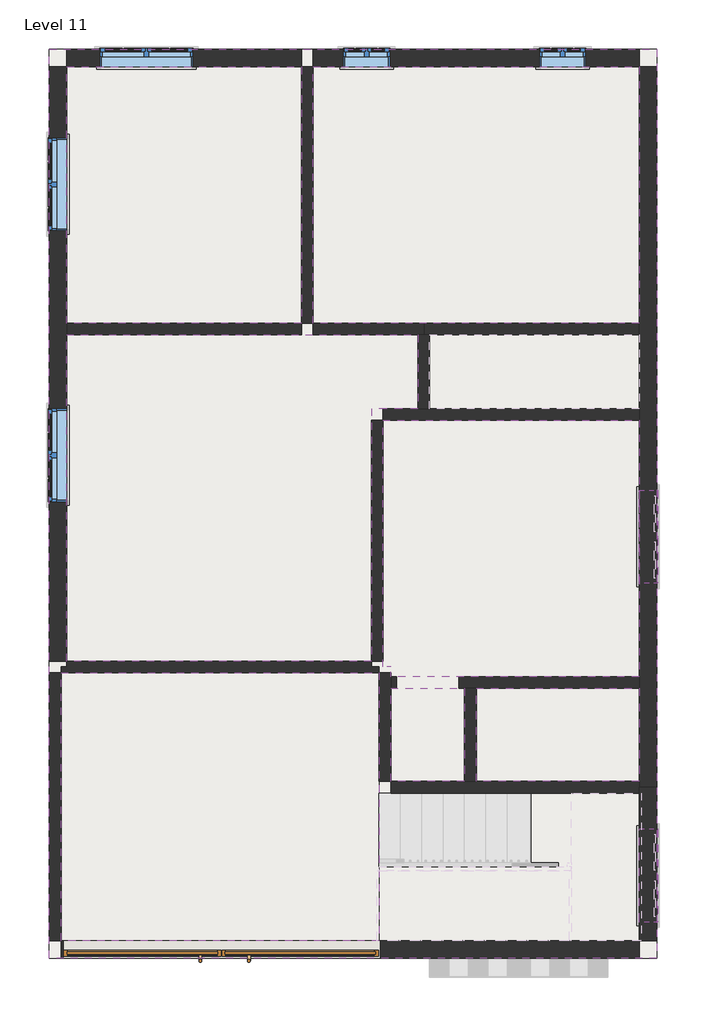
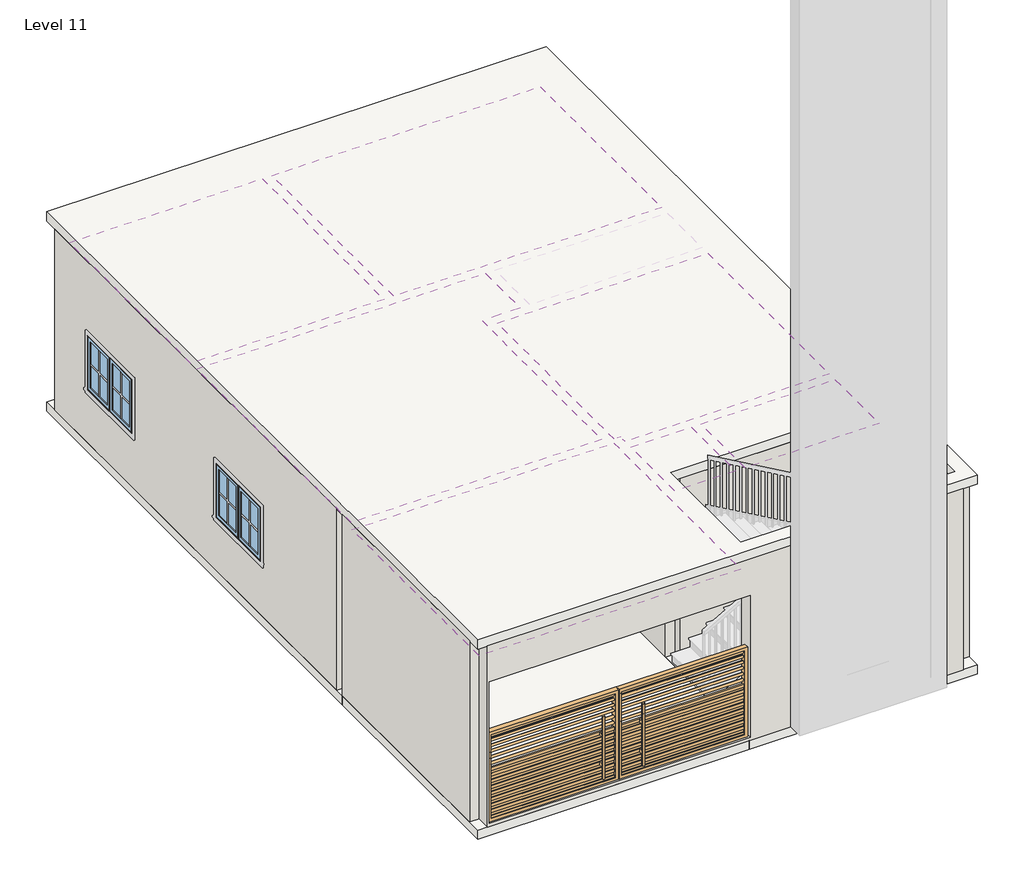
# One storey, part 1 of 3: 28 walls, 11 windows, 7 coverings, 3 slabs, 1 door.
"""IFC4 building model written with IfcOpenShell, lengths in millimetres."""

from ifc_helpers import new_model, si_unit, frame, origin, origin_with_axes, place, context, project, spatial, polyline, outline, extrude, faceted_brep, transform, mapped, element, save
from components import gate_gate_6d9155c2, window_casement_double_3_c417fced, window_casement_double_4_c19c33cb

model = new_model("IFC4")

# Units and contexts
model_context = context("Model", 3, world=origin())
ifc_project = project(units=[si_unit("LENGTHUNIT", "METRE", prefix="MILLI")], contexts=[model_context])

# Site, building, storey
site = spatial("IfcSite", under=ifc_project)
building = spatial("IfcBuilding", under=site)
storey = spatial("IfcBuildingStorey", under=building, Name="Level 11", Elevation=0.0)

# Coverings
placement = place(None, origin())
element("IfcCovering", 1, ObjectType="2' x 4' ACT System", at=placement, inside=storey, context=model_context, shape_type="SweptSolid", body=[
    extrude(outline(polyline([(-5680.5154463, 2323.8455275), (-5680.5154463, 5678.2330275), (-2607.1154463, 5678.2330275), (-2607.1154463, 2323.8455275), (-5680.5154463, 2323.8455275)])), frame((0.0, 0.0, 2743.2), z_axis=(0.0, 0.0, 1.0), x_axis=(1.0, 0.0, 0.0)), (0.0, 0.0, 1.0), 57.15),
])
element("IfcCovering", 2, ObjectType="2' x 4' ACT System", at=placement, inside=storey, context=model_context, shape_type="SweptSolid", body=[
    extrude(outline(polyline([(-2454.7154463, 2323.8455275), (-2454.7154463, 5678.2330275), (1812.4845537, 5678.2330275), (1812.4845537, 2323.8455275), (-2454.7154463, 2323.8455275)])), frame((0.0, 0.0, 2743.2), z_axis=(0.0, 0.0, 1.0), x_axis=(1.0, 0.0, 0.0)), (0.0, 0.0, 1.0), 57.15),
])
element("IfcCovering", 3, ObjectType="2' x 4' ACT System", at=placement, inside=storey, context=model_context, shape_type="SweptSolid", body=[
    extrude(outline(polyline([(-5680.5154463, -2095.7544725), (-5680.5154463, 2171.4455275), (-1083.1154463, 2171.4455275), (-1083.1154463, 1206.2455275), (-1692.7154463, 1206.2455275), (-1692.7154463, -2095.7544725), (-5680.5154463, -2095.7544725)])), frame((0.0, 0.0, 2743.2), z_axis=(0.0, 0.0, 1.0), x_axis=(1.0, 0.0, 0.0)), (0.0, 0.0, 1.0), 57.15),
])
element("IfcCovering", 4, ObjectType="2' x 4' ACT System", at=placement, inside=storey, context=model_context, shape_type="SweptSolid", body=[
    extrude(outline(polyline([(1812.4845537, 1053.8455275), (1812.4845537, -2298.9544725), (-1438.7154463, -2298.9544725), (-1438.7154463, -2171.9544725), (-1540.3154463, -2171.9544725), (-1540.3154463, 1053.8455275), (1812.4845537, 1053.8455275)])), frame((0.0, 0.0, 2743.2), z_axis=(0.0, 0.0, 1.0), x_axis=(1.0, 0.0, 0.0)), (0.0, 0.0, 1.0), 57.15),
])
element("IfcCovering", 5, ObjectType="2' x 4' ACT System", at=placement, inside=storey, context=model_context, shape_type="SweptSolid", body=[
    extrude(outline(polyline([(1812.4845537, -2451.3544725), (1812.4845537, -3670.5544725), (-321.1154463, -3670.5544725), (-321.1154463, -2451.3544725), (1812.4845537, -2451.3544725)])), frame((0.0, 0.0, 2743.2), z_axis=(0.0, 0.0, 1.0), x_axis=(1.0, 0.0, 0.0)), (0.0, 0.0, 1.0), 57.15),
])
element("IfcCovering", 6, ObjectType="2' x 4' ACT System", at=placement, inside=storey, context=model_context, shape_type="SweptSolid", body=[
    extrude(outline(polyline([(-473.5154463, -2451.3544725), (-473.5154463, -3670.5544725), (-1438.7154463, -3670.5544725), (-1438.7154463, -2451.3544725), (-473.5154463, -2451.3544725)])), frame((0.0, 0.0, 2743.2), z_axis=(0.0, 0.0, 1.0), x_axis=(1.0, 0.0, 0.0)), (0.0, 0.0, 1.0), 57.15),
])
element("IfcCovering", 7, ObjectType="2' x 4' ACT System", at=placement, inside=storey, context=model_context, shape_type="SweptSolid", body=[
    extrude(outline(polyline([(-1591.1154463, -2248.1544725), (-1591.1154463, -5753.3544725), (-5756.7154463, -5753.3544725), (-5756.7154463, -2248.1544725), (-1591.1154463, -2248.1544725)])), frame((0.0, 0.0, 2743.2), z_axis=(0.0, 0.0, 1.0), x_axis=(1.0, 0.0, 0.0)), (0.0, 0.0, 1.0), 57.15),
])

# Door
gate_gate_shape = gate_gate_6d9155c2(model_context)
element("IfcDoor", 8, ObjectType="GATE : GATE", at=placement, inside=storey, context=model_context, shape_type="MappedRepresentation", body=[
    mapped(gate_gate_shape, transform((0.0, 0.0, 0.0), x_axis=(1.0, 0.0, 0.0), y_axis=(0.0, 1.0, 0.0), z_axis=(0.0, 0.0, 1.0))),
])

# Slabs
element("IfcSlab", 9, ObjectType="Generic - 6\"", at=placement, inside=storey, context=model_context, shape_type="SweptSolid", body=[
    extrude(outline(polyline([(-5909.1154463, -2248.1544725), (-5909.1154463, 5906.8330275), (2041.0845537, 5906.8330275), (2041.0845537, -5981.9544725), (-1591.1154463, -5981.9544725), (-1591.1154463, -2248.1544725), (-5756.7154463, -2248.1544725), (-5909.1154463, -2248.1544725)])), frame((0.0, 0.0, -152.4), z_axis=(0.0, 0.0, 1.0), x_axis=(1.0, 0.0, 0.0)), (0.0, 0.0, 1.0), 152.4),
])
element("IfcSlab", 10, ObjectType="Generic - 6\"", at=placement, inside=storey, context=model_context, shape_type="SweptSolid", body=[
    extrude(outline(polyline([(-1591.1154463, -2248.1544725), (-1591.1154463, -5981.9544725), (-5909.1154463, -5981.9544725), (-5909.1154463, -2248.1544725), (-1591.1154463, -2248.1544725)])), frame((0.0, 0.0, -152.4), z_axis=(0.0, 0.0, 1.0), x_axis=(1.0, 0.0, 0.0)), (0.0, 0.0, 1.0), 152.4),
])
element("IfcSlab", 11, ObjectType="Generic - 6\"", at=placement, inside=storey, context=model_context, shape_type="SweptSolid", body=[
    extrude(outline(polyline([(2041.0845537, 5906.8330275), (2041.0845537, -5981.9544725), (-5909.1154463, -5981.9544725), (-5909.1154463, 5906.8330275), (2041.0845537, 5906.8330275)]), holes=[polyline([(1812.4845537, -3822.9544725), (-1591.1154463, -3822.9544725), (-1591.1154463, -5753.3544725), (1812.4845537, -5753.3544725), (1812.4845537, -3822.9544725)])]), frame((0.0, 0.0, 3048.0), z_axis=(0.0, 0.0, 1.0), x_axis=(1.0, 0.0, 0.0)), (0.0, 0.0, 1.0), 152.4),
])

# Walls
element("IfcWall", 12, ObjectType="Generic - 6\"", at=placement, inside=storey, context=model_context, shape_type="SweptSolid", body=[
    extrude(outline(polyline([(-5909.1154463, -5753.3544725), (-5909.1154463, -2248.1544725), (-5756.7154463, -2248.1544725), (-5756.7154463, -5753.3544725), (-5909.1154463, -5753.3544725)])), origin_with_axes(), (0.0, 0.0, 1.0), 3048.0),
])
element("IfcWall", 13, ObjectType="Generic - 6\"", at=placement, inside=storey, context=model_context, shape_type="Brep", body=[
    faceted_brep([(1812.4845537, -3670.5544725, 0.0), (-321.1154463, -3670.5544725, 0.0), (-473.5154463, -3670.5544725, 0.0), (-1438.7154463, -3670.5544725, 0.0), (-1438.7154463, -3670.5544725, 3048.0), (-473.5154463, -3670.5544725, 3048.0), (-321.1154463, -3670.5544725, 3048.0), (1812.4845537, -3670.5544725, 3048.0), (1812.4845537, -3822.9544725, 0.0), (1812.4845537, -3822.9544725, 3048.0), (-1438.7154463, -3822.9544725, 3048.0), (-1438.7154463, -3822.9544725, 0.0), (1812.4845537, -3746.7544725, 0.0), (1812.4845537, -3746.7544725, 3048.0)], [[[0, 1, 2, 3, 4, 5, 6, 7]], [[8, 9, 10, 11]], [[3, 2, 1, 0, 12, 8, 11]], [[7, 6, 5, 4, 10, 9, 13]], [[4, 3, 11, 10]], [[0, 7, 13, 9, 8, 12]]]),
])
element("IfcWall", 14, ObjectType="Generic - 6\"", at=placement, inside=storey, context=model_context, shape_type="Brep", body=[
    faceted_brep([(-1438.7154463, -3670.5544725, 0.0), (-1438.7154463, -2451.3544725, 0.0), (-1438.7154463, -2298.9544725, 0.0), (-1438.7154463, -2248.1544725, 0.0), (-1438.7154463, -2248.1544725, 3048.0), (-1438.7154463, -2298.9544725, 3048.0), (-1438.7154463, -2451.3544725, 3048.0), (-1438.7154463, -3670.5544725, 3048.0), (-1591.1154463, -3670.5544725, 0.0), (-1591.1154463, -3670.5544725, 3048.0), (-1591.1154463, -2248.1544725, 3048.0), (-1591.1154463, -2248.1544725, 0.0)], [[[0, 1, 2, 3, 4, 5, 6, 7]], [[8, 9, 10, 11]], [[3, 2, 1, 0, 8, 11]], [[7, 6, 5, 4, 10, 9]], [[0, 7, 9, 8]], [[4, 3, 11, 10]]]),
])
element("IfcWall", 15, ObjectType="Generic - 6\"", at=placement, inside=storey, context=model_context, shape_type="SweptSolid", body=[
    extrude(outline(polyline([(-5680.5154463, -2095.7544725), (-1692.7154463, -2095.7544725), (-1692.7154463, -2171.9544725), (-1591.1154463, -2171.9544725), (-1591.1154463, -2248.1544725), (-5756.7154463, -2248.1544725), (-5756.7154463, -2171.9544725), (-5680.5154463, -2171.9544725), (-5680.5154463, -2095.7544725)])), origin_with_axes(), (0.0, 0.0, 1.0), 3048.0),
])
element("IfcWall", 16, ObjectType="Generic - 6\"", at=placement, inside=storey, context=model_context, shape_type="Brep", body=[
    faceted_brep([(1812.4845537, -2451.3544725, 0.0), (1812.4845537, -2451.3544725, 3048.0), (-321.1154463, -2451.3544725, 3048.0), (-473.5154463, -2451.3544725, 3048.0), (-1438.7154463, -2451.3544725, 3048.0), (-1438.7154463, -2451.3544725, 0.0), (-1367.0206652, -2451.3544725, 0.0), (-1367.0206652, -2451.3544725, 2438.4), (-547.4818767, -2451.3544725, 2438.4), (-547.4818767, -2451.3544725, 0.0), (-473.5154463, -2451.3544725, 0.0), (-321.1154463, -2451.3544725, 0.0), (1812.4845537, -2298.9544725, 3048.0), (1812.4845537, -2298.9544725, 0.0), (-547.4818767, -2298.9544725, 0.0), (-547.4818767, -2298.9544725, 2438.4), (-1367.0206652, -2298.9544725, 2438.4), (-1367.0206652, -2298.9544725, 0.0), (-1438.7154463, -2298.9544725, 0.0), (-1438.7154463, -2298.9544725, 3048.0)], [[[0, 1, 2, 3, 4, 5, 6, 7, 8, 9, 10, 11]], [[12, 13, 14, 15, 16, 17, 18, 19]], [[5, 18, 17, 6]], [[13, 0, 11, 10, 9, 14]], [[4, 3, 2, 1, 12, 19]], [[1, 0, 13, 12]], [[5, 4, 19, 18]], [[7, 16, 15, 8]], [[16, 7, 6, 17]], [[8, 15, 14, 9]]]),
])
element("IfcWall", 17, ObjectType="Generic - 6\"", at=placement, inside=storey, context=model_context, shape_type="SweptSolid", body=[
    extrude(outline(polyline([(-321.1154463, -2451.3544725), (-321.1154463, -3670.5544725), (-473.5154463, -3670.5544725), (-473.5154463, -2451.3544725), (-321.1154463, -2451.3544725)])), origin_with_axes(), (0.0, 0.0, 1.0), 3048.0),
])
element("IfcWall", 18, ObjectType="Generic - 6\"", at=placement, inside=storey, context=model_context, shape_type="Brep", body=[
    faceted_brep([(-1540.3154463, -2095.7544725, 0.0), (-1540.3154463, 1053.8455275, 0.0), (-1540.3154463, 1053.8455275, 3048.0), (-1540.3154463, -2095.7544725, 3048.0), (-1692.7154463, -2095.7544725, 0.0), (-1692.7154463, -2095.7544725, 3048.0), (-1692.7154463, 1053.8455275, 3048.0), (-1692.7154463, 1053.8455275, 0.0), (-1591.1154463, -2095.7544725, 0.0), (-1591.1154463, -2095.7544725, 3048.0)], [[[0, 1, 2, 3]], [[4, 5, 6, 7]], [[1, 0, 8, 4, 7]], [[3, 2, 6, 5, 9]], [[0, 3, 9, 5, 4, 8]], [[2, 1, 7, 6]]]),
])
element("IfcWall", 19, ObjectType="Generic - 6\"", at=placement, inside=storey, context=model_context, shape_type="Brep", body=[
    faceted_brep([(-1540.3154463, 1053.8455275, 0.0), (1812.4845537, 1053.8455275, 0.0), (1812.4845537, 1053.8455275, 3048.0), (-1540.3154463, 1053.8455275, 3048.0), (-1540.3154463, 1206.2455275, 0.0), (-1540.3154463, 1206.2455275, 3048.0), (-1083.1154463, 1206.2455275, 3048.0), (-930.7154463, 1206.2455275, 3048.0), (1812.4845537, 1206.2455275, 3048.0), (1812.4845537, 1206.2455275, 0.0), (-930.7154463, 1206.2455275, 0.0), (-1083.1154463, 1206.2455275, 0.0)], [[[0, 1, 2, 3]], [[4, 5, 6, 7, 8, 9, 10, 11]], [[1, 0, 4, 11, 10, 9]], [[3, 2, 8, 7, 6, 5]], [[2, 1, 9, 8]], [[0, 3, 5, 4]]]),
])
element("IfcWall", 20, ObjectType="Generic - 6\"", at=placement, inside=storey, context=model_context, shape_type="Brep", body=[
    faceted_brep([(-930.7154463, 1206.2455275, 0.0), (-930.7154463, 2171.4455275, 0.0), (-930.7154463, 2171.4455275, 3048.0), (-930.7154463, 1206.2455275, 3048.0), (-1083.1154463, 1206.2455275, 0.0), (-1083.1154463, 1206.2455275, 3048.0), (-1083.1154463, 2171.4455275, 3048.0), (-1083.1154463, 2171.4455275, 0.0), (-1006.9154463, 2171.4455275, 0.0), (-1006.9154463, 2171.4455275, 3048.0)], [[[0, 1, 2, 3]], [[4, 5, 6, 7]], [[1, 0, 4, 7, 8]], [[3, 2, 9, 6, 5]], [[0, 3, 5, 4]], [[2, 1, 8, 7, 6, 9]]]),
])
element("IfcWall", 21, ObjectType="Generic - 6\"", at=placement, inside=storey, context=model_context, shape_type="Brep", body=[
    faceted_brep([(1812.4845537, 2323.8455275, 0.0), (-1006.9154463, 2323.8455275, 0.0), (-1006.9154463, 2323.8455275, 3048.0), (1812.4845537, 2323.8455275, 3048.0), (1812.4845537, 2171.4455275, 0.0), (1812.4845537, 2171.4455275, 3048.0), (-930.7154463, 2171.4455275, 3048.0), (-1006.9154463, 2171.4455275, 3048.0), (-1006.9154463, 2171.4455275, 0.0), (-930.7154463, 2171.4455275, 0.0)], [[[0, 1, 2, 3]], [[4, 5, 6, 7, 8, 9]], [[1, 0, 4, 9, 8]], [[2, 1, 8, 7]], [[3, 2, 7, 6, 5]], [[0, 3, 5, 4]]]),
])
element("IfcWall", 22, ObjectType="Generic - 6\"", at=placement, inside=storey, context=model_context, shape_type="Brep", body=[
    faceted_brep([(-2607.1154463, 5678.2330275, 0.0), (-2607.1154463, 2323.8455275, 0.0), (-2607.1154463, 2323.8455275, 3048.0), (-2607.1154463, 5678.2330275, 3048.0), (-2454.7154463, 5678.2330275, 0.0), (-2454.7154463, 5678.2330275, 3048.0), (-2454.7154463, 2323.8455275, 3048.0), (-2454.7154463, 2323.8455275, 0.0), (-2530.9154463, 5678.2330275, 0.0), (-2530.9154463, 2323.8455275, 0.0), (-2530.9154463, 2323.8455275, 3048.0), (-2530.9154463, 5678.2330275, 3048.0)], [[[0, 1, 2, 3]], [[4, 5, 6, 7]], [[1, 0, 8, 4, 7, 9]], [[3, 2, 10, 6, 5, 11]], [[0, 3, 11, 5, 4, 8]], [[2, 1, 9, 7, 6, 10]]]),
])
element("IfcWall", 23, ObjectType="Generic - 6\"", at=placement, inside=storey, context=model_context, shape_type="SweptSolid", body=[
    extrude(outline(polyline([(-5680.5154463, 2323.8455275), (-2607.1154463, 2323.8455275), (-2607.1154463, 2171.4455275), (-5680.5154463, 2171.4455275), (-5680.5154463, 2323.8455275)])), origin_with_axes(), (0.0, 0.0, 1.0), 3048.0),
])
element("IfcWall", 24, ObjectType="Generic - 6\"", at=placement, inside=storey, context=model_context, shape_type="Brep", body=[
    faceted_brep([(-1006.9154463, 2323.8455275, 0.0), (-2454.7154463, 2323.8455275, 0.0), (-2454.7154463, 2323.8455275, 3048.0), (-1006.9154463, 2323.8455275, 3048.0), (-1006.9154463, 2171.4455275, 0.0), (-1006.9154463, 2171.4455275, 3048.0), (-1083.1154463, 2171.4455275, 3048.0), (-2454.7154463, 2171.4455275, 3048.0), (-2454.7154463, 2171.4455275, 0.0), (-1083.1154463, 2171.4455275, 0.0)], [[[0, 1, 2, 3]], [[4, 5, 6, 7, 8, 9]], [[1, 0, 4, 9, 8]], [[3, 2, 7, 6, 5]], [[0, 3, 5, 4]], [[2, 1, 8, 7]]]),
])
element("IfcWall", 25, ObjectType="Generic - 6\"", at=placement, inside=storey, context=model_context, shape_type="SweptSolid", body=[
    extrude(outline(polyline([(-5680.5154463, -2095.7544725), (-1692.7154463, -2095.7544725), (-1692.7154463, -2171.9544725), (-1591.1154463, -2171.9544725), (-1591.1154463, -2248.1544725), (-5756.7154463, -2248.1544725), (-5756.7154463, -2171.9544725), (-5680.5154463, -2171.9544725), (-5680.5154463, -2095.7544725)])), origin_with_axes(), (0.0, 0.0, 1.0), 3048.0),
])
element("IfcWall", 26, ObjectType="Generic - 6\"", at=placement, inside=storey, context=model_context, shape_type="Brep", body=[
    faceted_brep([(-2607.1154463, 5678.2330275, 0.0), (-2607.1154463, 2323.8455275, 0.0), (-2607.1154463, 2323.8455275, 3048.0), (-2607.1154463, 5678.2330275, 3048.0), (-2454.7154463, 5678.2330275, 0.0), (-2454.7154463, 5678.2330275, 3048.0), (-2454.7154463, 2323.8455275, 3048.0), (-2454.7154463, 2323.8455275, 0.0), (-2530.9154463, 5678.2330275, 0.0), (-2530.9154463, 2323.8455275, 0.0), (-2530.9154463, 2323.8455275, 3048.0), (-2530.9154463, 5678.2330275, 3048.0)], [[[0, 1, 2, 3]], [[4, 5, 6, 7]], [[1, 0, 8, 4, 7, 9]], [[3, 2, 10, 6, 5, 11]], [[0, 3, 11, 5, 4, 8]], [[2, 1, 9, 7, 6, 10]]]),
])
element("IfcWall", 27, ObjectType="Generic - 6\"", at=placement, inside=storey, context=model_context, shape_type="SweptSolid", body=[
    extrude(outline(polyline([(-5680.5154463, 2323.8455275), (-2607.1154463, 2323.8455275), (-2607.1154463, 2171.4455275), (-5680.5154463, 2171.4455275), (-5680.5154463, 2323.8455275)])), origin_with_axes(), (0.0, 0.0, 1.0), 3048.0),
])
element("IfcWall", 28, ObjectType="Generic - 6\"", at=placement, inside=storey, context=model_context, shape_type="Brep", body=[
    faceted_brep([(-1006.9154463, 2323.8455275, 0.0), (-2454.7154463, 2323.8455275, 0.0), (-2454.7154463, 2323.8455275, 3048.0), (-1006.9154463, 2323.8455275, 3048.0), (-1006.9154463, 2171.4455275, 0.0), (-1006.9154463, 2171.4455275, 3048.0), (-1083.1154463, 2171.4455275, 3048.0), (-2454.7154463, 2171.4455275, 3048.0), (-2454.7154463, 2171.4455275, 0.0), (-1083.1154463, 2171.4455275, 0.0)], [[[0, 1, 2, 3]], [[4, 5, 6, 7, 8, 9]], [[1, 0, 4, 9, 8]], [[3, 2, 7, 6, 5]], [[0, 3, 5, 4]], [[2, 1, 8, 7]]]),
])
element("IfcWall", 29, ObjectType="Generic - 6\"", at=placement, inside=storey, context=model_context, shape_type="Brep", body=[
    faceted_brep([(-1438.7154463, -3822.9544725, 0.0), (1812.4845537, -3822.9544725, 0.0), (1812.4845537, -3822.9544725, 3048.0), (-1438.7154463, -3822.9544725, 3048.0), (-1438.7154463, -3670.5544725, 0.0), (-1438.7154463, -3670.5544725, 3048.0), (-473.5154463, -3670.5544725, 3048.0), (-321.1154463, -3670.5544725, 3048.0), (1812.4845537, -3670.5544725, 3048.0), (1812.4845537, -3670.5544725, 0.0), (-321.1154463, -3670.5544725, 0.0), (-473.5154463, -3670.5544725, 0.0), (1812.4845537, -3746.7544725, 0.0), (1812.4845537, -3746.7544725, 3048.0)], [[[0, 1, 2, 3]], [[4, 5, 6, 7, 8, 9, 10, 11]], [[1, 0, 4, 11, 10, 9, 12]], [[3, 2, 13, 8, 7, 6, 5]], [[2, 1, 12, 9, 8, 13]], [[0, 3, 5, 4]]]),
])
element("IfcWall", 30, ObjectType="Generic - 9\"", at=placement, inside=storey, context=model_context, shape_type="SweptSolid", body=[
    extrude(outline(polyline([(0.0, -5680.5154463), (0.0, -2607.1154463), (3048.0, -2607.1154463), (3048.0, -5680.5154463), (0.0, -5680.5154463)]), holes=[polyline([(1828.8, -4029.5154463), (914.4, -4029.5154463), (914.4, -5248.7154463), (1828.8, -5248.7154463), (1828.8, -4029.5154463)])]), frame((0.0, 5678.2330275, 0.0), z_axis=(0.0, 1.0, 0.0), x_axis=(0.0, 0.0, 1.0)), (0.0, 0.0, 1.0), 228.6),
])
element("IfcWall", 31, ObjectType="Generic - 9\"", at=placement, inside=storey, context=model_context, shape_type="Brep", body=[
    faceted_brep([(1812.4845537, 5678.2330275, 0.0), (1812.4845537, 2323.8455275, 0.0), (1812.4845537, 2171.4455275, 0.0), (1812.4845537, 1206.2455275, 0.0), (1812.4845537, 1053.8455275, 0.0), (1812.4845537, -2298.9544725, 0.0), (1812.4845537, -2451.3544725, 0.0), (1812.4845537, -3670.5544725, 0.0), (1812.4845537, -3746.7544725, 0.0), (1812.4845537, -3746.7544725, 3048.0), (1812.4845537, -3670.5544725, 3048.0), (1812.4845537, -2451.3544725, 3048.0), (1812.4845537, -2298.9544725, 3048.0), (1812.4845537, 1053.8455275, 3048.0), (1812.4845537, 1206.2455275, 3048.0), (1812.4845537, 2171.4455275, 3048.0), (1812.4845537, 2323.8455275, 3048.0), (1812.4845537, 5678.2330275, 3048.0), (1812.4845537, -1079.7544725, 2133.6), (1812.4845537, -1079.7544725, 1219.2), (1812.4845537, 139.4455275, 1219.2), (1812.4845537, 139.4455275, 2133.6), (2041.0845537, 5678.2330275, 0.0), (2041.0845537, 5678.2330275, 3048.0), (2041.0845537, -3746.7544725, 3048.0), (2041.0845537, -3746.7544725, 0.0), (2041.0845537, -1079.7544725, 2133.6), (2041.0845537, 139.4455275, 2133.6), (2041.0845537, 139.4455275, 1219.2), (2041.0845537, -1079.7544725, 1219.2)], [[[0, 1, 2, 3, 4, 5, 6, 7, 8, 9, 10, 11, 12, 13, 14, 15, 16, 17], [18, 19, 20, 21]], [[22, 23, 24, 25], [26, 27, 28, 29]], [[8, 7, 6, 5, 4, 3, 2, 1, 0, 22, 25]], [[9, 8, 25, 24]], [[17, 16, 15, 14, 13, 12, 11, 10, 9, 24, 23]], [[19, 18, 26, 29]], [[20, 19, 29, 28]], [[21, 20, 28, 27]], [[18, 21, 27, 26]], [[0, 17, 23, 22]]]),
])
element("IfcWall", 32, ObjectType="Generic - 9\"", at=placement, inside=storey, context=model_context, shape_type="SweptSolid", body=[
    extrude(outline(polyline([(0.0, -5756.7154463), (0.0, 1812.4845537), (3048.0, 1812.4845537), (3048.0, -5756.7154463), (0.0, -5756.7154463)]), holes=[polyline([(2438.4, -5729.1673724), (2438.4, -1576.8982041), (50.8, -1576.8982041), (50.8, -5729.1673724), (2438.4, -5729.1673724)])]), frame((0.0, -5981.9544725, 0.0), z_axis=(0.0, 1.0, 0.0), x_axis=(0.0, 0.0, 1.0)), (0.0, 0.0, 1.0), 228.6),
])
element("IfcWall", 33, ObjectType="Generic - 9\"", at=placement, inside=storey, context=model_context, shape_type="Brep", body=[
    faceted_brep([(-5909.1154463, 5678.2330275, 0.0), (-5909.1154463, -2095.7544725, 0.0), (-5909.1154463, -2095.7544725, 3048.0), (-5909.1154463, 5678.2330275, 3048.0), (-5909.1154463, 4751.1330275, 1828.8), (-5909.1154463, 3531.9330275, 1828.8), (-5909.1154463, 3531.9330275, 914.4), (-5909.1154463, 4751.1330275, 914.4), (-5909.1154463, 1206.2455275, 1828.8), (-5909.1154463, -12.9544725, 1828.8), (-5909.1154463, -12.9544725, 914.4), (-5909.1154463, 1206.2455275, 914.4), (-5680.5154463, 5678.2330275, 0.0), (-5680.5154463, 5678.2330275, 3048.0), (-5680.5154463, 2323.8455275, 3048.0), (-5680.5154463, 2171.4455275, 3048.0), (-5680.5154463, -2095.7544725, 3048.0), (-5680.5154463, -2095.7544725, 0.0), (-5680.5154463, 2171.4455275, 0.0), (-5680.5154463, 2323.8455275, 0.0), (-5680.5154463, 4751.1330275, 1828.8), (-5680.5154463, 4751.1330275, 914.4), (-5680.5154463, 3531.9330275, 914.4), (-5680.5154463, 3531.9330275, 1828.8), (-5680.5154463, 1206.2455275, 1828.8), (-5680.5154463, 1206.2455275, 914.4), (-5680.5154463, -12.9544725, 914.4), (-5680.5154463, -12.9544725, 1828.8)], [[[0, 1, 2, 3], [4, 5, 6, 7], [8, 9, 10, 11]], [[12, 13, 14, 15, 16, 17, 18, 19], [20, 21, 22, 23], [24, 25, 26, 27]], [[1, 0, 12, 19, 18, 17]], [[3, 2, 16, 15, 14, 13]], [[21, 20, 4, 7]], [[22, 21, 7, 6]], [[23, 22, 6, 5]], [[20, 23, 5, 4]], [[25, 24, 8, 11]], [[26, 25, 11, 10]], [[27, 26, 10, 9]], [[24, 27, 9, 8]], [[0, 3, 13, 12]], [[2, 1, 17, 16]]]),
])
element("IfcWall", 34, ObjectType="Generic - 9\"", at=placement, inside=storey, context=model_context, shape_type="SweptSolid", body=[
    extrude(outline(polyline([(0.0, -2454.7154463), (0.0, 1812.4845537), (3048.0, 1812.4845537), (3048.0, -2454.7154463), (0.0, -2454.7154463)]), holes=[polyline([(1828.8, -1451.4154463), (914.4, -1451.4154463), (914.4, -2061.0154463), (1828.8, -2061.0154463), (1828.8, -1451.4154463)]), polyline([(1828.8, 1113.9845537), (914.4, 1113.9845537), (914.4, 504.3845537), (1828.8, 504.3845537), (1828.8, 1113.9845537)])]), frame((0.0, 5678.2330275, 0.0), z_axis=(0.0, 1.0, 0.0), x_axis=(0.0, 0.0, 1.0)), (0.0, 0.0, 1.0), 228.6),
])
element("IfcWall", 35, ObjectType="Generic - 9\"", at=placement, inside=storey, context=model_context, shape_type="Brep", body=[
    faceted_brep([(1812.4845537, -3746.7544725, 0.0), (1812.4845537, -3822.9544725, 0.0), (1812.4845537, -5753.3544725, 0.0), (1812.4845537, -5753.3544725, 3048.0), (1812.4845537, -3822.9544725, 3048.0), (1812.4845537, -3746.7544725, 3048.0), (1812.4845537, -5512.0544725, 2133.6), (1812.4845537, -5512.0544725, 1219.2), (1812.4845537, -4292.8544725, 1219.2), (1812.4845537, -4292.8544725, 2133.6), (2041.0845537, -3746.7544725, 0.0), (2041.0845537, -3746.7544725, 3048.0), (2041.0845537, -5753.3544725, 3048.0), (2041.0845537, -5753.3544725, 0.0), (2041.0845537, -5512.0544725, 2133.6), (2041.0845537, -4292.8544725, 2133.6), (2041.0845537, -4292.8544725, 1219.2), (2041.0845537, -5512.0544725, 1219.2)], [[[0, 1, 2, 3, 4, 5], [6, 7, 8, 9]], [[10, 11, 12, 13], [14, 15, 16, 17]], [[2, 1, 0, 10, 13]], [[5, 4, 3, 12, 11]], [[0, 5, 11, 10]], [[6, 9, 15, 14]], [[9, 8, 16, 15]], [[8, 7, 17, 16]], [[7, 6, 14, 17]], [[3, 2, 13, 12]]]),
])
element("IfcWall", 36, ObjectType="Generic - 9\"", at=placement, inside=storey, context=model_context, shape_type="SweptSolid", body=[
    extrude(outline(polyline([(0.0, -5680.5154463), (0.0, -2607.1154463), (3048.0, -2607.1154463), (3048.0, -5680.5154463), (0.0, -5680.5154463)]), holes=[polyline([(1828.8, -4029.5154463), (914.4, -4029.5154463), (914.4, -5248.7154463), (1828.8, -5248.7154463), (1828.8, -4029.5154463)])]), frame((0.0, 5678.2330275, 0.0), z_axis=(0.0, 1.0, 0.0), x_axis=(0.0, 0.0, 1.0)), (0.0, 0.0, 1.0), 228.6),
])
element("IfcWall", 37, ObjectType="Generic - 9\"", at=placement, inside=storey, context=model_context, shape_type="SweptSolid", body=[
    extrude(outline(polyline([(0.0, -5756.7154463), (0.0, 1812.4845537), (3048.0, 1812.4845537), (3048.0, -5756.7154463), (0.0, -5756.7154463)]), holes=[polyline([(2438.4, -5729.1673724), (2438.4, -1576.8982041), (50.8, -1576.8982041), (50.8, -5729.1673724), (2438.4, -5729.1673724)])]), frame((0.0, -5981.9544725, 0.0), z_axis=(0.0, 1.0, 0.0), x_axis=(0.0, 0.0, 1.0)), (0.0, 0.0, 1.0), 228.6),
])
element("IfcWall", 38, ObjectType="Generic - 9\"", at=placement, inside=storey, context=model_context, shape_type="SweptSolid", body=[
    extrude(outline(polyline([(0.0, -2454.7154463), (0.0, 1812.4845537), (3048.0, 1812.4845537), (3048.0, -2454.7154463), (0.0, -2454.7154463)]), holes=[polyline([(1828.8, -1451.4154463), (914.4, -1451.4154463), (914.4, -2061.0154463), (1828.8, -2061.0154463), (1828.8, -1451.4154463)]), polyline([(1828.8, 1113.9845537), (914.4, 1113.9845537), (914.4, 504.3845537), (1828.8, 504.3845537), (1828.8, 1113.9845537)])]), frame((0.0, 5678.2330275, 0.0), z_axis=(0.0, 1.0, 0.0), x_axis=(0.0, 0.0, 1.0)), (0.0, 0.0, 1.0), 228.6),
])
element("IfcWall", 39, ObjectType="Generic - 9\"", at=placement, inside=storey, context=model_context, shape_type="SweptSolid", body=[
    extrude(outline(polyline([(-3822.9544725, 0.0), (-5753.3544725, 0.0), (-5753.3544725, 3048.0), (-3822.9544725, 3048.0), (-3822.9544725, 0.0)]), holes=[polyline([(-5512.0544725, 2133.6), (-5512.0544725, 1219.2), (-4292.8544725, 1219.2), (-4292.8544725, 2133.6), (-5512.0544725, 2133.6)])]), frame((1812.4845537, 0.0, 0.0), z_axis=(1.0, 0.0, 0.0), x_axis=(0.0, 1.0, 0.0)), (0.0, 0.0, 1.0), 228.6),
])

# Windows
window_casement_double_3_shape = window_casement_double_3_c417fced(model_context)
element("IfcWindow", 40, ObjectType="Window-Casement-Double : 3'", at=placement, inside=storey, context=model_context, shape_type="MappedRepresentation", body=[
    mapped(window_casement_double_3_shape, transform((-1756.2154463, 5792.5330275, 0.0), x_axis=(1.0, 0.0, 0.0), y_axis=(0.0, 1.0, 0.0), z_axis=(0.0, 0.0, 1.0))),
])
element("IfcWindow", 41, ObjectType="Window-Casement-Double : 3'", at=placement, inside=storey, context=model_context, shape_type="MappedRepresentation", body=[
    mapped(window_casement_double_3_shape, transform((809.1845537, 5792.5330275, 0.0), x_axis=(1.0, 0.0, 0.0), y_axis=(0.0, 1.0, 0.0), z_axis=(0.0, 0.0, 1.0))),
])
element("IfcWindow", 42, ObjectType="Window-Casement-Double : 3'", at=placement, inside=storey, context=model_context, shape_type="MappedRepresentation", body=[
    mapped(window_casement_double_3_shape, transform((-1756.2154463, 5792.5330275, 0.0), x_axis=(1.0, 0.0, 0.0), y_axis=(0.0, 1.0, 0.0), z_axis=(0.0, 0.0, 1.0))),
])
element("IfcWindow", 43, ObjectType="Window-Casement-Double : 3'", at=placement, inside=storey, context=model_context, shape_type="MappedRepresentation", body=[
    mapped(window_casement_double_3_shape, transform((809.1845537, 5792.5330275, 0.0), x_axis=(1.0, 0.0, 0.0), y_axis=(0.0, 1.0, 0.0), z_axis=(0.0, 0.0, 1.0))),
])
window_casement_double_4_shape = window_casement_double_4_c19c33cb(model_context)
element("IfcWindow", 44, ObjectType="Window-Casement-Double : 4'", at=placement, inside=storey, context=model_context, shape_type="MappedRepresentation", body=[
    mapped(window_casement_double_4_shape, transform((-4639.1154463, 5792.5330275, 0.0), x_axis=(1.0, 0.0, 0.0), y_axis=(0.0, 1.0, 0.0), z_axis=(0.0, 0.0, 1.0))),
])
element("IfcWindow", 45, ObjectType="Window-Casement-Double : 4'", at=placement, inside=storey, context=model_context, shape_type="MappedRepresentation", body=[
    mapped(window_casement_double_4_shape, transform((-5794.8154463, 4141.5330275, 0.0), x_axis=(0.0, 1.0, 0.0), y_axis=(-1.0, 0.0, 0.0), z_axis=(0.0, 0.0, 1.0))),
])
element("IfcWindow", 46, ObjectType="Window-Casement-Double : 4'", at=placement, inside=storey, context=model_context, shape_type="MappedRepresentation", body=[
    mapped(window_casement_double_4_shape, transform((-5794.8154463, 596.6455275, 0.0), x_axis=(0.0, 1.0, 0.0), y_axis=(-1.0, 0.0, 0.0), z_axis=(0.0, 0.0, 1.0))),
])
element("IfcWindow", 47, ObjectType="Window-Casement-Double : 4'", at=placement, inside=storey, context=model_context, shape_type="MappedRepresentation", body=[
    mapped(window_casement_double_4_shape, transform((1926.7845537, -470.1544725, 304.8), x_axis=(0.0, -1.0, 0.0), y_axis=(1.0, 0.0, 0.0), z_axis=(0.0, 0.0, 1.0))),
])
element("IfcWindow", 48, ObjectType="Window-Casement-Double : 4'", at=placement, inside=storey, context=model_context, shape_type="MappedRepresentation", body=[
    mapped(window_casement_double_4_shape, transform((1926.7845537, -4902.4544725, 304.8), x_axis=(0.0, -1.0, 0.0), y_axis=(1.0, 0.0, 0.0), z_axis=(0.0, 0.0, 1.0))),
])
element("IfcWindow", 49, ObjectType="Window-Casement-Double : 4'", at=placement, inside=storey, context=model_context, shape_type="MappedRepresentation", body=[
    mapped(window_casement_double_4_shape, transform((-4639.1154463, 5792.5330275, 0.0), x_axis=(1.0, 0.0, 0.0), y_axis=(0.0, 1.0, 0.0), z_axis=(0.0, 0.0, 1.0))),
])
element("IfcWindow", 50, ObjectType="Window-Casement-Double : 4'", at=placement, inside=storey, context=model_context, shape_type="MappedRepresentation", body=[
    mapped(window_casement_double_4_shape, transform((1926.7845537, -4902.4544725, 304.8), x_axis=(0.0, -1.0, 0.0), y_axis=(1.0, 0.0, 0.0), z_axis=(0.0, 0.0, 1.0))),
])

save(model, "model.ifc")

# Revit data of these elements
# Type "2' x 4' ACT System"
#   Assembly Code = "C3030210"
#   built-in parameter 1002203 = 1 (stored number, unit not read)
#   built-in parameter 1002202 = 1 (stored number, unit not read)
#   Layers, outside or top first: 0' - 1 5/8" "Default" (function 1); 0' - 0 5/8" "Acoustic Ceiling Tile 24 x 48" (function 5)
# Type "GATE : GATE"
#   Type Mark = "11"
# Type "Generic - 6\""
#   Assembly Code = "B1010"
#   Function = 0
#   Layers, outside or top first: 0' - 6" no material (function 1)
# Type "Generic - 6\""
#   Assembly Code = "B2010"
#   Layers, outside or top first: 0' - 6" no material (function 1)
# Type "Generic - 9\""
#   Assembly Code = "B2010"
#   Layers, outside or top first: 0' - 9" no material (function 1)
# Type "Window-Casement-Double : 3'"
#   Type Mark = "19"
#   Fire Rating = "0.5h"
#   Assembly Code = "B2020100"
#   Analytic Construction = "Double glazing - domestic"
#   Frame Extension [instance default] = 0' - 0 1/4"
#   Window Inset [instance default] = 0' - 0"
#   Wall Thickness [instance default] = 0' - 6"
#   Interior Wall Closure [instance default] = 0' - 2 1/4"
#   Half Width = 1' - 0"
#   Visual Light Transmittance = 0.81
#   Thermal Resistance (R) = 1.8146 (h·ft²·°F)/BTU
#   Solar Heat Gain Coefficient = 0.76
#   Rough Width = 2' - 0 1/2"
#   Rough Height = 3' - 0 1/2"
#   Height = 3' - 0"
#   Heat Transfer Coefficient (U) = 0.5511 BTU/(h·ft²·°F)
#   Exterior Wall Closure [instance default] = 0' - 1 1/4"
#   Extension Jamb [instance default] = 0' - 2 1/4"
#   Default Sill Height = 3' - 0"
#   Width = 2' - 0"
#   Muntin Visibility = yes
#   Interior Trim Visibility [instance default] = yes
#   Exterior Trim Visibility [instance default] = yes
#   Extension Jamb Visibility [instance default] = yes
#   Interior Trim Material = Wood - Stained
#   Muntin Pattern = Muntin Pattern_2x2 : Muntin Pattern_2x2
#   Interior Trim = Trim-Window-Interior-Flat : Picture Frame
#   Interior Frame Material = Wood - Stained
#   Glass Panel Material = Glass
#   Exterior Trim Material = Clad - White
#   Exterior Trim = Trim-Window-Exterior-Flat : with Sill
#   Exterior Frame Material = Clad - White
#   Wall Closure = (empty or 0)
# Type "Window-Casement-Double : 4'"
#   Type Mark = "18"
#   Fire Rating = "0.5h"
#   Assembly Code = "B2020100"
#   Analytic Construction = "Double glazing - domestic"
#   Frame Extension [instance default] = 0' - 0 1/4"
#   Window Inset [instance default] = 0' - 0"
#   Wall Thickness [instance default] = 0' - 6"
#   Interior Wall Closure [instance default] = 0' - 2 1/4"
#   Half Width = 2' - 0"
#   Visual Light Transmittance = 0.81
#   Thermal Resistance (R) = 1.8146 (h·ft²·°F)/BTU
#   Solar Heat Gain Coefficient = 0.76
#   Rough Width = 4' - 0 1/2"
#   Rough Height = 3' - 0 1/2"
#   Height = 3' - 0"
#   Heat Transfer Coefficient (U) = 0.5511 BTU/(h·ft²·°F)
#   Exterior Wall Closure [instance default] = 0' - 1 1/4"
#   Extension Jamb [instance default] = 0' - 2 1/4"
#   Default Sill Height = 3' - 0"
#   Width = 4' - 0"
#   Muntin Visibility = yes
#   Interior Trim Visibility [instance default] = yes
#   Exterior Trim Visibility [instance default] = yes
#   Extension Jamb Visibility [instance default] = yes
#   Interior Trim Material = Wood - Stained
#   Muntin Pattern = Muntin Pattern_2x2 : Muntin Pattern_2x2
#   Interior Trim = Trim-Window-Interior-Flat : Picture Frame
#   Interior Frame Material = Wood - Stained
#   Glass Panel Material = Glass
#   Exterior Trim Material = Clad - White
#   Exterior Trim = Trim-Window-Exterior-Flat : with Sill
#   Exterior Frame Material = Clad - White
#   Wall Closure = (empty or 0)
# Elements 1, 2, 3, 4, 5, 6, 7 (IfcCovering, "2' x 4' ACT System")
#   Height Offset From Level = 9' - 0"
#   Phase Created = New Construction
#   Materials on its faces: "Acoustic Ceiling Tile 24 x 48", "Default"
# Element 8 (IfcDoor, "GATE : GATE")
#   Phase Created = New Construction
#   Materials on its faces: "Door - Panel", "Iron, Ductile", "Aluminum"
# Element 9 (IfcSlab, "Generic - 6\"")
#   built-in parameter 1001955 = -1.5708 (stored number, unit not read)
#   Height Offset From Level = 0' - 0"
#   Phase Created = New Construction
#   Materials on its faces: "Default Floor", "TILE"
# Element 10 (IfcSlab, "Generic - 6\"")
#   Height Offset From Level = 0' - 0"
#   Phase Created = New Construction
#   Materials on its faces: "Default Floor", "Grass"
# Element 11 (IfcSlab, "Generic - 6\"")
#   Height Offset From Level = 10' - 6"
#   Phase Created = New Construction
#   Materials on its faces: "Default Floor"
# Element 12 (IfcWall, "Generic - 6\"")
#   Top Offset = 0' - 0"
#   Base Offset = 0' - 0"
#   Unconnected Height = 10' - 0"
#   wall height = 10' - 0"
#   Phase Created = New Construction
#   Base Constraint = Level 11
#   Materials on its faces: "Default Wall", "WALL PAINT 4"
# Element 13 (IfcWall, "Generic - 6\"")
#   Top Offset = 0' - 0"
#   Base Offset = 0' - 0"
#   Unconnected Height = 10' - 0"
#   wall height = 10' - 0"
#   Phase Created = New Construction
#   Base Constraint = Level 11
#   Materials on its faces: "Default Wall", "WALL PAINT 5", "MARBLE"
# Element 14 (IfcWall, "Generic - 6\"")
#   Top Offset = 0' - 0"
#   Base Offset = 0' - 0"
#   Unconnected Height = 10' - 0"
#   wall height = 10' - 0"
#   Phase Created = New Construction
#   Base Constraint = Level 11
#   Materials on its faces: "Default Wall", "WALL PAINT 4", "MARBLE"
# Elements 15, 25 (IfcWall, "Generic - 6\"")
#   Top Offset = 0' - 0"
#   Base Offset = 0' - 0"
#   Unconnected Height = 10' - 0"
#   wall height = 10' - 0"
#   Phase Created = New Construction
#   Base Constraint = Level 11
#   Materials on its faces: "Default Wall", "WALL PAINT 2", "MARBLE"
# Elements 16, 19 (IfcWall, "Generic - 6\"")
#   Top Offset = 0' - 0"
#   Base Offset = 0' - 0"
#   Unconnected Height = 10' - 0"
#   wall height = 10' - 0"
#   Phase Created = New Construction
#   Base Constraint = Level 11
#   Materials on its faces: "Default Wall", "WALL PAINT 4", "WALL PAINT 5"
# Element 17 (IfcWall, "Generic - 6\"")
#   Top Offset = 0' - 0"
#   Base Offset = 0' - 0"
#   Unconnected Height = 10' - 0"
#   wall height = 10' - 0"
#   Phase Created = New Construction
#   Base Constraint = Level 11
#   Materials on its faces: "Default Wall", "WALL PAINT 5"
# Element 18 (IfcWall, "Generic - 6\"")
#   Top Offset = 0' - 0"
#   Base Offset = 0' - 0"
#   Unconnected Height = 10' - 0"
#   wall height = 10' - 0"
#   Phase Created = New Construction
#   Base Constraint = Level 11
#   Materials on its faces: "Default Wall", "WALL PAINT 4", "WALL PAINT 2"
# Element 20 (IfcWall, "Generic - 6\"")
#   Top Offset = 0' - 0"
#   Base Offset = 0' - 0"
#   Unconnected Height = 10' - 0"
#   wall height = 10' - 0"
#   Phase Created = New Construction
#   Base Constraint = Level 11
#   Materials on its faces: "Default Wall", "WALL PAINT 5", "WALL PAINT 2"
# Element 21 (IfcWall, "Generic - 6\"")
#   Top Offset = 0' - 0"
#   Base Offset = 0' - 0"
#   Unconnected Height = 10' - 0"
#   wall height = 10' - 0"
#   Phase Created = New Construction
#   Base Constraint = Level 11
#   Materials on its faces: "Default Wall", "WALL PAINT 3", "WALL PAINT 5"
# Elements 22, 26 (IfcWall, "Generic - 6\"")
#   Top Offset = 0' - 0"
#   Base Offset = 0' - 0"
#   Unconnected Height = 10' - 0"
#   wall height = 10' - 0"
#   Phase Created = New Construction
#   Base Constraint = Level 11
#   Materials on its faces: "Default Wall", "WALL PAINT 1", "WALL PAINT 3"
# Elements 23, 27 (IfcWall, "Generic - 6\"")
#   Top Offset = 0' - 0"
#   Base Offset = 0' - 0"
#   Unconnected Height = 10' - 0"
#   wall height = 10' - 0"
#   Phase Created = New Construction
#   Base Constraint = Level 11
#   Materials on its faces: "Default Wall", "WALL PAINT 1", "WALL PAINT 2"
# Elements 24, 28 (IfcWall, "Generic - 6\"")
#   Top Offset = 0' - 0"
#   Base Offset = 0' - 0"
#   Unconnected Height = 10' - 0"
#   wall height = 10' - 0"
#   Phase Created = New Construction
#   Base Constraint = Level 11
#   Materials on its faces: "Default Wall", "WALL PAINT 3", "WALL PAINT 2"
# Element 29 (IfcWall, "Generic - 6\"")
#   Top Offset = 0' - 0"
#   Base Offset = 0' - 0"
#   Unconnected Height = 10' - 0"
#   wall height = 10' - 0"
#   Phase Created = New Construction
#   Base Constraint = Level 11
#   Materials on its faces: "Default Wall"
# Elements 30, 36 (IfcWall, "Generic - 9\"")
#   Top Offset = 0' - 0"
#   Base Offset = 0' - 0"
#   Unconnected Height = 10' - 0"
#   wall height = 10' - 0"
#   Phase Created = New Construction
#   Base Constraint = Level 11
#   Materials on its faces: "Default Wall", "WALL PAINT 1"
# Elements 31, 33 (IfcWall, "Generic - 9\"")
#   Top Offset = 0' - 0"
#   Base Offset = 0' - 0"
#   Unconnected Height = 10' - 0"
#   wall height = 10' - 0"
#   Phase Created = New Construction
#   Base Constraint = Level 11
#   Materials on its faces: "Default Wall"
# Elements 32, 35, 37, 39 (IfcWall, "Generic - 9\"")
#   Top Offset = 0' - 0"
#   Base Offset = 0' - 0"
#   Unconnected Height = 10' - 0"
#   wall height = 10' - 0"
#   Phase Created = New Construction
#   Base Constraint = Level 11
#   Materials on its faces: "Default Wall", "WALL PAINT 4"
# Elements 34, 38 (IfcWall, "Generic - 9\"")
#   Top Offset = 0' - 0"
#   Base Offset = 0' - 0"
#   Unconnected Height = 10' - 0"
#   wall height = 10' - 0"
#   Phase Created = New Construction
#   Base Constraint = Level 11
#   Materials on its faces: "Default Wall", "WALL PAINT 3"
# Element 40 (IfcWindow, "Window-Casement-Double : 3'")
#   Mark = "19"
#   Window Inset = 0' - 0"
#   Interior Wall Closure = 0' - 2 1/4"
#   Frame Extension = 0' - 0 1/4"
#   Exterior Wall Closure = 0' - 1 1/4"
#   Interior Trim Visibility = yes
#   Exterior Trim Visibility = yes
#   Phase Created = New Construction
#   Materials on its faces: "Wood - Stained", "Glass", "Clad - White"
# Element 41 (IfcWindow, "Window-Casement-Double : 3'")
#   Mark = "20"
#   Window Inset = 0' - 0"
#   Interior Wall Closure = 0' - 2 1/4"
#   Frame Extension = 0' - 0 1/4"
#   Exterior Wall Closure = 0' - 1 1/4"
#   Interior Trim Visibility = yes
#   Exterior Trim Visibility = yes
#   Phase Created = New Construction
#   Materials on its faces: "Wood - Stained", "Glass", "Clad - White"
# Element 42 (IfcWindow, "Window-Casement-Double : 3'")
#   Mark = "25"
#   Window Inset = 0' - 0"
#   Interior Wall Closure = 0' - 2 1/4"
#   Frame Extension = 0' - 0 1/4"
#   Exterior Wall Closure = 0' - 1 1/4"
#   Interior Trim Visibility = yes
#   Exterior Trim Visibility = yes
#   Phase Created = New Construction
#   Materials on its faces: "Wood - Stained", "Glass", "Clad - White"
# Element 43 (IfcWindow, "Window-Casement-Double : 3'")
#   Mark = "26"
#   Window Inset = 0' - 0"
#   Interior Wall Closure = 0' - 2 1/4"
#   Frame Extension = 0' - 0 1/4"
#   Exterior Wall Closure = 0' - 1 1/4"
#   Interior Trim Visibility = yes
#   Exterior Trim Visibility = yes
#   Phase Created = New Construction
#   Materials on its faces: "Wood - Stained", "Glass", "Clad - White"
# Element 44 (IfcWindow, "Window-Casement-Double : 4'")
#   Mark = "14"
#   Window Inset = 0' - 0"
#   Interior Wall Closure = 0' - 2 1/4"
#   Frame Extension = 0' - 0 1/4"
#   Exterior Wall Closure = 0' - 1 1/4"
#   Interior Trim Visibility = yes
#   Exterior Trim Visibility = yes
#   Phase Created = New Construction
#   Materials on its faces: "Wood - Stained", "Glass", "Clad - White"
# Element 45 (IfcWindow, "Window-Casement-Double : 4'")
#   Mark = "15"
#   Window Inset = 0' - 0"
#   Interior Wall Closure = 0' - 2 1/4"
#   Frame Extension = 0' - 0 1/4"
#   Exterior Wall Closure = 0' - 1 1/4"
#   Interior Trim Visibility = yes
#   Exterior Trim Visibility = yes
#   Phase Created = New Construction
#   Materials on its faces: "Wood - Stained", "Glass", "Clad - White"
# Element 46 (IfcWindow, "Window-Casement-Double : 4'")
#   Mark = "16"
#   Window Inset = 0' - 0"
#   Interior Wall Closure = 0' - 2 1/4"
#   Frame Extension = 0' - 0 1/4"
#   Exterior Wall Closure = 0' - 1 1/4"
#   Interior Trim Visibility = yes
#   Exterior Trim Visibility = yes
#   Phase Created = New Construction
#   Materials on its faces: "Wood - Stained", "Glass", "Clad - White"
# Element 47 (IfcWindow, "Window-Casement-Double : 4'")
#   Mark = "17"
#   Window Inset = 0' - 0"
#   Interior Wall Closure = 0' - 2 1/4"
#   Frame Extension = 0' - 0 1/4"
#   Exterior Wall Closure = 0' - 1 1/4"
#   Interior Trim Visibility = yes
#   Exterior Trim Visibility = yes
#   Phase Created = New Construction
#   Materials on its faces: "Wood - Stained", "Glass", "Clad - White"
# Element 48 (IfcWindow, "Window-Casement-Double : 4'")
#   Mark = "18"
#   Window Inset = 0' - 0"
#   Interior Wall Closure = 0' - 2 1/4"
#   Frame Extension = 0' - 0 1/4"
#   Exterior Wall Closure = 0' - 1 1/4"
#   Interior Trim Visibility = yes
#   Exterior Trim Visibility = yes
#   Phase Created = New Construction
#   Materials on its faces: "Wood - Stained", "Glass", "Clad - White"
# Element 49 (IfcWindow, "Window-Casement-Double : 4'")
#   Mark = "23"
#   Window Inset = 0' - 0"
#   Interior Wall Closure = 0' - 2 1/4"
#   Frame Extension = 0' - 0 1/4"
#   Exterior Wall Closure = 0' - 1 1/4"
#   Interior Trim Visibility = yes
#   Exterior Trim Visibility = yes
#   Phase Created = New Construction
#   Materials on its faces: "Wood - Stained", "Glass", "Clad - White"
# Element 50 (IfcWindow, "Window-Casement-Double : 4'")
#   Mark = "24"
#   Window Inset = 0' - 0"
#   Interior Wall Closure = 0' - 2 1/4"
#   Frame Extension = 0' - 0 1/4"
#   Exterior Wall Closure = 0' - 1 1/4"
#   Interior Trim Visibility = yes
#   Exterior Trim Visibility = yes
#   Phase Created = New Construction
#   Materials on its faces: "Wood - Stained", "Glass", "Clad - White"
# Materials
#   "Default": colour RGB 127 127 127, transparency 0, Cost = 0
#   "Acoustic Ceiling Tile 24 x 48": class "Generic", colour RGB 229 229 229, transparency 0, Description = "Acoustic Ceiling Tile 24 x 48", Cost = 0
#   "Wood - Stained": class "Wood", colour RGB 224 178 126, transparency 0, Cost = 0
#   "Glass": class "Glass", colour RGB 0 128 192, transparency 0.75, Description = "Soda Lime Glass", Cost = 0
#   "Clad - White": class "Wood", colour RGB 242 242 238, transparency 0, Cost = 0
#   "Door - Panel": class "Wood", colour RGB 210 159 95, transparency 0, Cost = 0
#   "Iron, Ductile": class "Metal", colour RGB 0 0 0, transparency 0, Description = "Ductile cast iron", Cost = 0
#   "Aluminum": class "Metal", colour RGB 247 247 247, transparency 0, Description = "Aluminum 6061", Cost = 0
#   "Default Floor": colour RGB 128 128 128, transparency 0, Cost = 0
#   "TILE": class "Generic", colour RGB 120 120 120, transparency 0, Cost = 0
#   "Grass": class "Generic", colour RGB 104 137 66, transparency 0, Description = "Physical material.", Cost = 0
#   "Default Wall": colour RGB 128 128 128, transparency 0, Cost = 0
#   "WALL PAINT 4": class "Generic", colour RGB 120 120 120, transparency 0, Cost = 0
#   "WALL PAINT 5": class "Generic", colour RGB 120 120 120, transparency 0, Cost = 0
#   "MARBLE": class "Generic", colour RGB 120 120 120, transparency 0, Cost = 0
#   "WALL PAINT 2": class "Generic", colour RGB 120 120 120, transparency 0, Cost = 0
#   "WALL PAINT 3": class "Generic", colour RGB 120 120 120, transparency 0, Cost = 0
#   "WALL PAINT 1": class "Generic", colour RGB 120 120 120, transparency 0, Cost = 0
